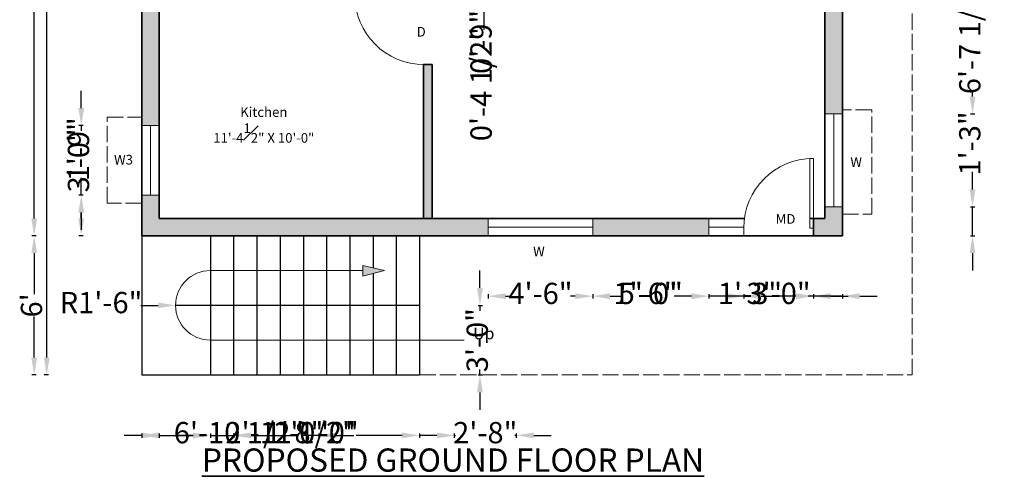
# Model space of a CAD drawing. Units: inches. Extents: x 2339 to 2848, y 489 to 1121.
# Tile 1 of 3: x 2339 to 2848, y 489 to 725. Entities that reach past the tile are written whole.
import ezdxf

# ---------------------------------------------------------------- set-up
doc = ezdxf.new("R2010")
doc.units = ezdxf.units.IN
doc.linetypes.add('ACAD_ISO02W100', pattern=[15, 12, -3])
for name, color, linetype, lineweight in [('A-ANNO-DIMS', 2, 'Continuous', 18), ('A-ANNO-SYMB', 7, 'Continuous', 18), ('A-ANNO-TEXT', 7, 'Continuous', 18), ('A-ANNO-TITL', 7, 'Continuous', 35), ('A-AREA-IDEN', 7, 'Continuous', 18), ('A-DOOR', 3, 'Continuous', 18), ('A-FLOR-STRS', 7, 'Continuous', 25), ('A-GLAZ', 4, 'Continuous', 18), ('A-ROOF-OVHD', 8, 'ACAD_ISO02W100', 13), ('A-WALL', 7, 'Continuous', 35), ('C-PROP', 8, 'ACAD_ISO02W100', 18)]:
    doc.layers.add(name, color=color, linetype=linetype, lineweight=lineweight)
doc.layers.add('A-WALL-PATT', color=18, linetype='Continuous', lineweight=13, true_color=0x000000)
doc.styles.get("Standard").update_dxf_attribs({"font": 'arial.ttf'})
doc.dimstyles.new('ISO-25', dxfattribs={"dimtxt": 11, "dimasz": 9, "dimexe": 1.25, "dimexo": 0.625, "dimtad": 0, "dimlunit": 4, "dimtxsty": 'Standard', "dimcen": 2.5, "dimadec": 0, "dimazin": 0, "dimtfac": 1, "dimtmove": 0, "dimatfit": 3, "dimfxl": 1, "dimfxlon": 1, "dimfrac": 1, "dimarcsym": 0})

# ---------------------------------------------------------------- blocks, each defined once
blk = doc.blocks.new('*U2')
for p, q in [((0, 0), (0, -4)), ((36, 0), (36, -4))]:
    blk.add_line(p, q)
blk.add_lwpolyline([(0, 0), (0, 36), (1.75, 36), (1.75, 0)], close=True)
blk.add_arc((0, 0), 36, 0, 90)
blk = doc.blocks.new('*D4')
at = {"layer": 'A-ANNO-DIMS', "color": 0, "lineweight": -2, "transparency": 16777216}
for p, q in [((2347.8, 1057.44), (2345.55, 1057.44)), ((2346.8, 1048.44), (2346.8, 845.39)), ((2346.8, 622.44), (2346.8, 825.48)), ((2347.8, 613.44), (2345.55, 613.44))]:
    blk.add_line(p, q, dxfattribs=at)
at = {"layer": 'A-ANNO-DIMS', "color": 0, "transparency": 16777216}
for points in [[(2345.3, 1048.44), (2348.3, 1048.44), (2346.8, 1057.44)], [(2345.3, 622.44), (2348.3, 622.44), (2346.8, 613.44)]]:
    blk.add_solid(points, dxfattribs=at)
at = {"layer": 'Defpoints', "color": 0, "transparency": 16777216}
for p in [(2402.35, 1057.44), (2346.8, 613.44), (2402.35, 613.44)]:
    blk.add_point(p, dxfattribs=at)
at = {"layer": 'A-ANNO-DIMS', "color": 0, "transparency": 16777216, "insert": (2346.8, 835.44), "char_height": 11, "attachment_point": 5, "rotation": 90}
blk.add_mtext("37'", dxfattribs=at)
blk = doc.blocks.new('*D5')
at = {"layer": 'A-ANNO-DIMS', "color": 0, "lineweight": -2, "transparency": 16777216}
for p, q in [((2347.8, 613.44), (2345.55, 613.44)), ((2346.8, 604.44), (2346.8, 583.15)), ((2346.8, 550.44), (2346.8, 571.72)), ((2347.8, 541.44), (2345.55, 541.44))]:
    blk.add_line(p, q, dxfattribs=at)
at = {"layer": 'A-ANNO-DIMS', "color": 0, "transparency": 16777216}
for points in [[(2345.3, 604.44), (2348.3, 604.44), (2346.8, 613.44)], [(2345.3, 550.44), (2348.3, 550.44), (2346.8, 541.44)]]:
    blk.add_solid(points, dxfattribs=at)
at = {"layer": 'Defpoints', "color": 0, "transparency": 16777216}
for p in [(2402.35, 613.44), (2346.8, 541.44), (2402.35, 541.44)]:
    blk.add_point(p, dxfattribs=at)
at = {"layer": 'A-ANNO-DIMS', "color": 0, "transparency": 16777216, "insert": (2346.8, 577.44), "char_height": 11, "attachment_point": 5, "rotation": 90}
blk.add_mtext("6'", dxfattribs=at)
blk = doc.blocks.new('WIN-48IN')
for p, q in [((0, 0), (0, 9)), ((48, 0), (48, 9)), ((0, 4.5), (48, 4.5))]:
    blk.add_line(p, q)
blk = doc.blocks.new('*D11')
at = {"layer": 'A-ANNO-DIMS', "color": 0, "lineweight": -2, "transparency": 16777216}
for p, q in [((2354.26, 1082.3), (2352.01, 1082.3)), ((2353.26, 1073.3), (2353.26, 831.61)), ((2353.26, 550.44), (2353.26, 792.13)), ((2354.26, 541.44), (2352.01, 541.44))]:
    blk.add_line(p, q, dxfattribs=at)
at = {"layer": 'A-ANNO-DIMS', "color": 0, "transparency": 16777216}
for points in [[(2351.76, 1073.3), (2354.76, 1073.3), (2353.26, 1082.3)], [(2351.76, 550.44), (2354.76, 550.44), (2353.26, 541.44)]]:
    blk.add_solid(points, dxfattribs=at)
at = {"layer": 'Defpoints', "color": 0, "transparency": 16777216}
for p in [(2353.26, 1082.3), (2493.85, 1082.3), (2402.35, 541.44)]:
    blk.add_point(p, dxfattribs=at)
at = {"layer": 'A-ANNO-DIMS', "color": 0, "transparency": 16777216, "insert": (2353.26, 811.87), "char_height": 11, "attachment_point": 5, "rotation": 90}
blk.add_mtext('45\'-1"', dxfattribs=at)
blk = doc.blocks.new('*D12')
at = {"layer": 'A-ANNO-DIMS', "color": 0, "lineweight": -2, "transparency": 16777216}
for p, q in [((2402.35, 511.19), (2402.35, 508.94)), ((2411.35, 510.19), (2428.85, 510.19)), ((2437.85, 511.19), (2437.85, 508.94)), ((2437.85, 510.19), (2446.85, 510.19))]:
    blk.add_line(p, q, dxfattribs=at)
at = {"layer": 'A-ANNO-DIMS', "color": 0, "transparency": 16777216}
for points in [[(2411.35, 511.69), (2411.35, 508.69), (2402.35, 510.19)], [(2428.85, 511.69), (2428.85, 508.69), (2437.85, 510.19)]]:
    blk.add_solid(points, dxfattribs=at)
at = {"layer": 'Defpoints', "color": 0, "transparency": 16777216}
for p in [(2402.35, 541.44), (2437.85, 541.44), (2437.85, 510.19)]:
    blk.add_point(p, dxfattribs=at)
at = {"layer": 'A-ANNO-DIMS', "color": 0, "transparency": 16777216, "insert": (2479.27, 510.19), "char_height": 11, "attachment_point": 5}
blk.add_mtext('2\'-11 1/2"', dxfattribs=at)
blk = doc.blocks.new('*D13')
at = {"layer": 'A-ANNO-DIMS', "color": 0, "lineweight": -2, "transparency": 16777216}
for p, q in [((2428.85, 510.19), (2419.85, 510.19)), ((2437.85, 511.19), (2437.85, 508.94)), ((2437.85, 510.19), (2449.85, 510.19)), ((2449.85, 511.19), (2449.85, 508.94)), ((2458.85, 510.19), (2467.85, 510.19))]:
    blk.add_line(p, q, dxfattribs=at)
at = {"layer": 'A-ANNO-DIMS', "color": 0, "transparency": 16777216}
for points in [[(2428.85, 511.69), (2428.85, 508.69), (2437.85, 510.19)], [(2458.85, 511.69), (2458.85, 508.69), (2449.85, 510.19)]]:
    blk.add_solid(points, dxfattribs=at)
at = {"layer": 'Defpoints', "color": 0, "transparency": 16777216}
for p in [(2437.85, 541.44), (2449.85, 541.44), (2449.85, 510.19)]:
    blk.add_point(p, dxfattribs=at)
at = {"layer": 'A-ANNO-DIMS', "color": 0, "transparency": 16777216, "insert": (2482.57, 510.19), "char_height": 11, "attachment_point": 5}
blk.add_mtext('1\'-0"', dxfattribs=at)
blk = doc.blocks.new('*D14')
at = {"layer": 'A-ANNO-DIMS', "color": 0, "lineweight": -2, "transparency": 16777216}
for p, q in [((2449.85, 511.19), (2449.85, 508.94)), ((2458.85, 510.19), (2482.59, 510.19)), ((2536.85, 510.19), (2513.1, 510.19)), ((2545.85, 511.19), (2545.85, 508.94))]:
    blk.add_line(p, q, dxfattribs=at)
at = {"layer": 'A-ANNO-DIMS', "color": 0, "transparency": 16777216}
for points in [[(2458.85, 511.69), (2458.85, 508.69), (2449.85, 510.19)], [(2536.85, 511.69), (2536.85, 508.69), (2545.85, 510.19)]]:
    blk.add_solid(points, dxfattribs=at)
at = {"layer": 'Defpoints', "color": 0, "transparency": 16777216}
for p in [(2449.85, 541.44), (2545.85, 541.44), (2545.85, 510.19)]:
    blk.add_point(p, dxfattribs=at)
at = {"layer": 'A-ANNO-DIMS', "color": 0, "transparency": 16777216, "insert": (2497.85, 510.19), "char_height": 11, "attachment_point": 5}
blk.add_mtext('8\'-0"', dxfattribs=at)
blk = doc.blocks.new('*D15')
at = {"layer": 'A-ANNO-DIMS', "color": 0, "lineweight": -2, "transparency": 16777216}
for p, q in [((2581.35, 583.19), (2581.35, 580.94)), ((2590.35, 582.19), (2592.88, 582.19)), ((2626.35, 582.19), (2623.81, 582.19)), ((2635.35, 583.19), (2635.35, 580.94))]:
    blk.add_line(p, q, dxfattribs=at)
at = {"layer": 'A-ANNO-DIMS', "color": 0, "transparency": 16777216}
for points in [[(2590.35, 583.69), (2590.35, 580.69), (2581.35, 582.19)], [(2626.35, 583.69), (2626.35, 580.69), (2635.35, 582.19)]]:
    blk.add_solid(points, dxfattribs=at)
at = {"layer": 'Defpoints', "color": 0, "transparency": 16777216}
for p in [(2581.35, 613.44), (2635.35, 613.44), (2581.35, 582.19)]:
    blk.add_point(p, dxfattribs=at)
at = {"layer": 'A-ANNO-DIMS', "color": 0, "transparency": 16777216, "insert": (2608.35, 582.19), "char_height": 11, "attachment_point": 5}
blk.add_mtext('4\'-6"', dxfattribs=at)
blk = doc.blocks.new('*D16')
at = {"layer": 'A-ANNO-DIMS', "color": 0, "lineweight": -2, "transparency": 16777216}
for p, q in [((2635.35, 583.19), (2635.35, 580.94)), ((2644.35, 582.19), (2650.1, 582.19)), ((2686.35, 582.19), (2680.59, 582.19)), ((2695.35, 583.19), (2695.35, 580.94))]:
    blk.add_line(p, q, dxfattribs=at)
at = {"layer": 'A-ANNO-DIMS', "color": 0, "transparency": 16777216}
for points in [[(2644.35, 583.69), (2644.35, 580.69), (2635.35, 582.19)], [(2686.35, 583.69), (2686.35, 580.69), (2695.35, 582.19)]]:
    blk.add_solid(points, dxfattribs=at)
at = {"layer": 'Defpoints', "color": 0, "transparency": 16777216}
for p in [(2635.35, 613.44), (2695.35, 613.44), (2635.35, 582.19)]:
    blk.add_point(p, dxfattribs=at)
at = {"layer": 'A-ANNO-DIMS', "color": 0, "transparency": 16777216, "insert": (2665.35, 582.19), "char_height": 11, "attachment_point": 5}
blk.add_mtext('5\'-0"', dxfattribs=at)
blk = doc.blocks.new('*D17')
at = {"layer": 'A-ANNO-DIMS', "color": 0, "lineweight": -2, "transparency": 16777216}
for p, q in [((2686.35, 582.19), (2677.35, 582.19)), ((2695.35, 583.19), (2695.35, 580.94)), ((2713.35, 582.19), (2695.35, 582.19)), ((2713.35, 583.19), (2713.35, 580.94)), ((2722.35, 582.19), (2731.35, 582.19))]:
    blk.add_line(p, q, dxfattribs=at)
at = {"layer": 'A-ANNO-DIMS', "color": 0, "transparency": 16777216}
for points in [[(2686.35, 583.69), (2686.35, 580.69), (2695.35, 582.19)], [(2722.35, 583.69), (2722.35, 580.69), (2713.35, 582.19)]]:
    blk.add_solid(points, dxfattribs=at)
at = {"layer": 'Defpoints', "color": 0, "transparency": 16777216}
for p in [(2695.35, 613.44), (2713.35, 613.44), (2695.35, 582.19)]:
    blk.add_point(p, dxfattribs=at)
at = {"layer": 'A-ANNO-DIMS', "color": 0, "transparency": 16777216, "insert": (2662.62, 582.19), "char_height": 11, "attachment_point": 5}
blk.add_mtext('1\'-6"', dxfattribs=at)
blk = doc.blocks.new('*D18')
at = {"layer": 'A-ANNO-DIMS', "color": 0, "lineweight": -2, "transparency": 16777216}
for p, q in [((2704.35, 582.19), (2695.35, 582.19)), ((2713.35, 583.19), (2713.35, 580.94)), ((2713.35, 582.19), (2716.11, 582.19)), ((2749.35, 582.19), (2746.59, 582.19)), ((2749.35, 583.19), (2749.35, 580.94)), ((2758.35, 582.19), (2767.35, 582.19))]:
    blk.add_line(p, q, dxfattribs=at)
at = {"layer": 'A-ANNO-DIMS', "color": 0, "transparency": 16777216}
for points in [[(2704.35, 583.69), (2704.35, 580.69), (2713.35, 582.19)], [(2758.35, 583.69), (2758.35, 580.69), (2749.35, 582.19)]]:
    blk.add_solid(points, dxfattribs=at)
at = {"layer": 'Defpoints', "color": 0, "transparency": 16777216}
for p in [(2713.35, 613.44), (2749.35, 613.44), (2713.35, 582.19)]:
    blk.add_point(p, dxfattribs=at)
at = {"layer": 'A-ANNO-DIMS', "color": 0, "transparency": 16777216, "insert": (2731.35, 582.19), "char_height": 11, "attachment_point": 5}
blk.add_mtext('3\'-0"', dxfattribs=at)
blk = doc.blocks.new('*D19')
at = {"layer": 'A-ANNO-DIMS', "color": 0, "lineweight": -2, "transparency": 16777216}
for p, q in [((2740.35, 582.19), (2731.35, 582.19)), ((2749.35, 583.19), (2749.35, 580.94)), ((2764.35, 582.19), (2749.35, 582.19)), ((2764.35, 583.19), (2764.35, 580.94)), ((2773.35, 582.19), (2782.35, 582.19))]:
    blk.add_line(p, q, dxfattribs=at)
at = {"layer": 'A-ANNO-DIMS', "color": 0, "transparency": 16777216}
for points in [[(2740.35, 583.69), (2740.35, 580.69), (2749.35, 582.19)], [(2773.35, 583.69), (2773.35, 580.69), (2764.35, 582.19)]]:
    blk.add_solid(points, dxfattribs=at)
at = {"layer": 'Defpoints', "color": 0, "transparency": 16777216}
for p in [(2749.35, 613.44), (2764.35, 613.44), (2749.35, 582.19)]:
    blk.add_point(p, dxfattribs=at)
at = {"layer": 'A-ANNO-DIMS', "color": 0, "transparency": 16777216, "insert": (2716.62, 582.19), "char_height": 11, "attachment_point": 5}
blk.add_mtext('1\'-3"', dxfattribs=at)
blk = doc.blocks.new('*D20')
at = {"layer": 'A-ANNO-DIMS', "color": 0, "lineweight": -2, "transparency": 16777216}
for p, q in [((2371.1, 634.44), (2371.1, 643.44)), ((2372.1, 634.44), (2369.85, 634.44)), ((2371.1, 622.44), (2371.1, 625.44)), ((2372.1, 613.44), (2369.85, 613.44))]:
    blk.add_line(p, q, dxfattribs=at)
at = {"layer": 'A-ANNO-DIMS', "color": 0, "transparency": 16777216}
for points in [[(2369.6, 625.44), (2372.6, 625.44), (2371.1, 634.44)], [(2369.6, 622.44), (2372.6, 622.44), (2371.1, 613.44)]]:
    blk.add_solid(points, dxfattribs=at)
at = {"layer": 'Defpoints', "color": 0, "transparency": 16777216}
for p in [(2371.1, 634.44), (2402.35, 634.44), (2402.35, 613.44)]:
    blk.add_point(p, dxfattribs=at)
at = {"layer": 'A-ANNO-DIMS', "color": 0, "transparency": 16777216, "insert": (2371.1, 658.17), "char_height": 11, "attachment_point": 5, "rotation": 90}
blk.add_mtext('1\'-9"', dxfattribs=at)
blk = doc.blocks.new('*D21')
at = {"layer": 'A-ANNO-DIMS', "color": 0, "lineweight": -2, "transparency": 16777216}
for p, q in [((2371.1, 679.44), (2371.1, 688.44)), ((2372.1, 670.44), (2369.85, 670.44)), ((2371.1, 670.44), (2371.1, 667.68)), ((2371.1, 634.44), (2371.1, 637.2)), ((2372.1, 634.44), (2369.85, 634.44)), ((2371.1, 625.44), (2371.1, 616.44))]:
    blk.add_line(p, q, dxfattribs=at)
at = {"layer": 'A-ANNO-DIMS', "color": 0, "transparency": 16777216}
for points in [[(2369.6, 679.44), (2372.6, 679.44), (2371.1, 670.44)], [(2369.6, 625.44), (2372.6, 625.44), (2371.1, 634.44)]]:
    blk.add_solid(points, dxfattribs=at)
at = {"layer": 'Defpoints', "color": 0, "transparency": 16777216}
for p in [(2371.1, 670.44), (2402.35, 670.44), (2402.35, 634.44)]:
    blk.add_point(p, dxfattribs=at)
at = {"layer": 'A-ANNO-DIMS', "color": 0, "transparency": 16777216, "insert": (2371.1, 652.44), "char_height": 11, "attachment_point": 5, "rotation": 90}
blk.add_mtext('3\'-0"', dxfattribs=at)
blk = doc.blocks.new('*D27')
at = {"layer": 'A-ANNO-DIMS', "color": 0, "lineweight": -2, "transparency": 16777216}
for p, q in [((2402.35, 510.19), (2393.35, 510.19)), ((2411.35, 511.19), (2411.35, 508.94)), ((2411.35, 510.19), (2420.23, 510.19)), ((2493.85, 510.19), (2484.96, 510.19)), ((2493.85, 511.19), (2493.85, 508.94)), ((2502.85, 510.19), (2511.85, 510.19))]:
    blk.add_line(p, q, dxfattribs=at)
at = {"layer": 'A-ANNO-DIMS', "color": 0, "transparency": 16777216}
for points in [[(2402.35, 511.69), (2402.35, 508.69), (2411.35, 510.19)], [(2502.85, 511.69), (2502.85, 508.69), (2493.85, 510.19)]]:
    blk.add_solid(points, dxfattribs=at)
at = {"layer": 'Defpoints', "color": 0, "transparency": 16777216}
for p in [(2411.35, 1048.44), (2493.85, 1048.44), (2493.85, 510.19)]:
    blk.add_point(p, dxfattribs=at)
at = {"layer": 'A-ANNO-DIMS', "color": 0, "transparency": 16777216, "insert": (2452.6, 510.19), "char_height": 11, "attachment_point": 5}
blk.add_mtext('6\'-10 1/2"', dxfattribs=at)
blk = doc.blocks.new('*D31')
at = {"layer": 'A-ANNO-DIMS', "color": 0, "lineweight": -2, "transparency": 16777216}
for p, q in [((2831.6, 637.44), (2831.6, 646.44)), ((2830.6, 628.44), (2832.85, 628.44)), ((2831.6, 613.44), (2831.6, 628.44)), ((2830.6, 613.44), (2832.85, 613.44)), ((2831.6, 604.44), (2831.6, 595.44))]:
    blk.add_line(p, q, dxfattribs=at)
at = {"layer": 'A-ANNO-DIMS', "color": 0, "transparency": 16777216}
for points in [[(2830.1, 637.44), (2833.1, 637.44), (2831.6, 628.44)], [(2830.1, 604.44), (2833.1, 604.44), (2831.6, 613.44)]]:
    blk.add_solid(points, dxfattribs=at)
at = {"layer": 'Defpoints', "color": 0, "transparency": 16777216}
for p in [(2764.35, 628.44), (2831.6, 628.44), (2764.35, 613.44)]:
    blk.add_point(p, dxfattribs=at)
at = {"layer": 'A-ANNO-DIMS', "color": 0, "transparency": 16777216, "insert": (2831.6, 661.17), "char_height": 11, "attachment_point": 5, "rotation": 90}
blk.add_mtext('1\'-3"', dxfattribs=at)
blk = doc.blocks.new('*D32')
at = {"layer": 'A-ANNO-DIMS', "color": 0, "lineweight": -2, "transparency": 16777216}
for p, q in [((2830.6, 755.94), (2832.85, 755.94)), ((2831.6, 746.94), (2831.6, 744.28)), ((2831.6, 685.44), (2831.6, 688.1)), ((2830.6, 676.44), (2832.85, 676.44))]:
    blk.add_line(p, q, dxfattribs=at)
at = {"layer": 'A-ANNO-DIMS', "color": 0, "transparency": 16777216}
for points in [[(2830.1, 746.94), (2833.1, 746.94), (2831.6, 755.94)], [(2830.1, 685.44), (2833.1, 685.44), (2831.6, 676.44)]]:
    blk.add_solid(points, dxfattribs=at)
at = {"layer": 'Defpoints', "color": 0, "transparency": 16777216}
for p in [(2764.35, 755.94), (2831.6, 755.94), (2764.35, 676.44)]:
    blk.add_point(p, dxfattribs=at)
at = {"layer": 'A-ANNO-DIMS', "color": 0, "transparency": 16777216, "insert": (2831.6, 716.19), "char_height": 11, "attachment_point": 5, "rotation": 90}
blk.add_mtext('6\'-7 1/2"', dxfattribs=at)
blk = doc.blocks.new('*D36')
at = {"layer": 'A-ANNO-DIMS', "color": 0, "lineweight": -2, "transparency": 16777216}
for p, q in [((2554.85, 510.19), (2545.85, 510.19)), ((2563.85, 511.19), (2563.85, 508.94)), ((2563.85, 510.19), (2564.51, 510.19)), ((2595.85, 510.19), (2595.19, 510.19)), ((2595.85, 511.19), (2595.85, 508.94)), ((2604.85, 510.19), (2613.85, 510.19))]:
    blk.add_line(p, q, dxfattribs=at)
at = {"layer": 'A-ANNO-DIMS', "color": 0, "transparency": 16777216}
for points in [[(2554.85, 511.69), (2554.85, 508.69), (2563.85, 510.19)], [(2604.85, 511.69), (2604.85, 508.69), (2595.85, 510.19)]]:
    blk.add_solid(points, dxfattribs=at)
at = {"layer": 'Defpoints', "color": 0, "transparency": 16777216}
for p in [(2563.85, 971.94), (2595.85, 971.94), (2595.85, 510.19)]:
    blk.add_point(p, dxfattribs=at)
at = {"layer": 'A-ANNO-DIMS', "color": 0, "transparency": 16777216, "insert": (2579.85, 510.19), "char_height": 11, "attachment_point": 5}
blk.add_mtext('2\'-8"', dxfattribs=at)
blk = doc.blocks.new('*D41')
at = {"layer": 'A-ANNO-DIMS', "color": 0, "lineweight": -2, "transparency": 16777216}
for p, q in [((2577.1, 586.44), (2577.1, 595.44)), ((2576.1, 577.44), (2578.35, 577.44)), ((2577.1, 577.44), (2577.1, 574.68)), ((2576.1, 541.44), (2578.35, 541.44)), ((2577.1, 541.44), (2577.1, 544.2)), ((2577.1, 532.44), (2577.1, 523.44))]:
    blk.add_line(p, q, dxfattribs=at)
at = {"layer": 'A-ANNO-DIMS', "color": 0, "transparency": 16777216}
for points in [[(2575.6, 586.44), (2578.6, 586.44), (2577.1, 577.44)], [(2575.6, 532.44), (2578.6, 532.44), (2577.1, 541.44)]]:
    blk.add_solid(points, dxfattribs=at)
at = {"layer": 'Defpoints', "color": 0, "transparency": 16777216}
for p in [(2545.85, 577.44), (2545.85, 541.44), (2577.1, 541.44)]:
    blk.add_point(p, dxfattribs=at)
at = {"layer": 'A-ANNO-DIMS', "color": 0, "transparency": 16777216, "insert": (2577.1, 559.44), "char_height": 11, "attachment_point": 5, "rotation": 90}
blk.add_mtext('3\'-0"', dxfattribs=at)
blk = doc.blocks.new('*D45')
at = {"layer": 'A-ANNO-DIMS', "color": 0, "lineweight": -2, "transparency": 16777216}
for p, q in [((2579.1, 764.94), (2579.1, 773.94)), ((2578.1, 755.94), (2580.35, 755.94)), ((2579.1, 755.94), (2579.1, 746.94)), ((2578.1, 746.94), (2580.35, 746.94)), ((2579.1, 737.94), (2579.1, 728.94))]:
    blk.add_line(p, q, dxfattribs=at)
at = {"layer": 'A-ANNO-DIMS', "color": 0, "transparency": 16777216}
for points in [[(2577.6, 764.94), (2580.6, 764.94), (2579.1, 755.94)], [(2577.6, 737.94), (2580.6, 737.94), (2579.1, 746.94)]]:
    blk.add_solid(points, dxfattribs=at)
at = {"layer": 'Defpoints', "color": 0, "transparency": 16777216}
for p in [(2547.85, 755.94), (2547.85, 746.94), (2579.1, 746.94)]:
    blk.add_point(p, dxfattribs=at)
at = {"layer": 'A-ANNO-DIMS', "color": 0, "transparency": 16777216, "insert": (2579.1, 713.69), "char_height": 11, "attachment_point": 5, "rotation": 90}
blk.add_mtext('0\'-9"', dxfattribs=at)
blk = doc.blocks.new('*D46')
at = {"layer": 'A-ANNO-DIMS', "color": 0, "lineweight": -2, "transparency": 16777216}
for p, q in [((2579.1, 751.44), (2579.1, 760.44)), ((2578.1, 742.44), (2580.35, 742.44)), ((2578.1, 737.94), (2580.35, 737.94)), ((2579.1, 742.44), (2579.1, 737.94)), ((2579.1, 728.94), (2579.1, 719.94))]:
    blk.add_line(p, q, dxfattribs=at)
at = {"layer": 'A-ANNO-DIMS', "color": 0, "transparency": 16777216}
for points in [[(2577.6, 751.44), (2580.6, 751.44), (2579.1, 742.44)], [(2577.6, 728.94), (2580.6, 728.94), (2579.1, 737.94)]]:
    blk.add_solid(points, dxfattribs=at)
at = {"layer": 'Defpoints', "color": 0, "transparency": 16777216}
for p in [(2547.85, 742.44), (2547.85, 737.94), (2579.1, 737.94)]:
    blk.add_point(p, dxfattribs=at)
at = {"layer": 'A-ANNO-DIMS', "color": 0, "transparency": 16777216, "insert": (2579.1, 691.88), "char_height": 11, "attachment_point": 5, "rotation": 90}
blk.add_mtext('0\'-4 1/2"', dxfattribs=at)
blk = doc.blocks.new('*D48')
at = {"layer": 'A-ANNO-DIMS', "color": 0, "lineweight": -2, "transparency": 16777216}
for p, q in [((2401.85, 577.44), (2410.85, 577.44)), ((2437.85, 577.44), (2419.85, 577.44))]:
    blk.add_line(p, q, dxfattribs=at)
at = {"layer": 'A-ANNO-DIMS', "color": 0, "transparency": 16777216}
blk.add_solid([(2410.85, 578.94), (2410.85, 575.94), (2419.85, 577.44)], dxfattribs=at)
at = {"layer": 'Defpoints', "color": 0, "transparency": 16777216}
for p in [(2419.85, 577.44), (2437.85, 577.44)]:
    blk.add_point(p, dxfattribs=at)
at = {"layer": 'A-ANNO-DIMS', "color": 0, "transparency": 16777216, "insert": (2381.34, 577.44), "char_height": 11, "attachment_point": 5, "rotation": 359.9991}
blk.add_mtext('R1\'-6"', dxfattribs=at)

msp = doc.modelspace()

# ---------------------------------------------------------------- hatches: boundary and pattern name
at = {"layer": 'A-ANNO-SYMB'}
h = msp.add_hatch(color=256, dxfattribs=at)
h.dxf.hatch_style = 1
h.paths.add_polyline_path([(2516.636, 597.983), (2516.636, 592.471), (2527.847, 595.438)])
at = {"layer": 'A-WALL-PATT'}
h = msp.add_hatch(color=256, dxfattribs=at)
h.dxf.hatch_style = 1
h.paths.add_polyline_path([(2493.847, 1057.438), (2402.347, 1057.438), (2402.347, 991.938), (2411.347, 991.938), (2411.347, 1048.438), (2493.847, 1048.438)])
h.paths.add_polyline_path([(2411.347, 931.938), (2402.347, 931.938), (2402.347, 912.438), (2411.347, 912.438), (2411.347, 918.438)])
h.paths.add_polyline_path([(2411.347, 871.438), (2411.347, 877.438), (2402.347, 877.438), (2402.347, 803.938), (2411.347, 803.938)])
h.paths.add_polyline_path([(2547.847, 871.438), (2411.347, 871.438), (2411.347, 866.938), (2547.847, 866.938)])
h.paths.add_polyline_path([(2447.347, 922.938), (2411.347, 922.938), (2411.347, 918.438), (2447.347, 918.438)])
h.paths.add_polyline_path([(2552.347, 866.938), (2547.847, 866.938), (2547.847, 791.938), (2552.347, 791.938)])
h.paths.add_polyline_path([(2411.347, 755.938), (2402.347, 755.938), (2402.347, 670.438), (2411.347, 670.438)])
h.paths.add_polyline_path([(2552.347, 755.938), (2547.847, 755.938), (2547.847, 746.938), (2411.347, 746.938), (2411.347, 742.438), (2547.847, 742.438), (2547.847, 737.938), (2552.347, 737.938)])
h.paths.add_polyline_path([(2552.347, 701.938), (2547.847, 701.938), (2547.847, 622.438), (2552.347, 622.438)])
h.paths.add_polyline_path([(2581.347, 622.438), (2411.347, 622.438), (2411.347, 634.438), (2402.347, 634.438), (2402.347, 613.438), (2581.347, 613.438)])
h.paths.add_polyline_path([(2695.347, 622.438), (2635.347, 622.438), (2635.347, 613.438), (2695.347, 613.438)])
h.paths.add_polyline_path([(2764.347, 628.438), (2755.347, 628.438), (2755.347, 622.438), (2749.347, 622.438), (2749.347, 613.438), (2764.347, 613.438)])
h.paths.add_polyline_path([(2764.347, 755.938), (2760.347, 755.938), (2755.347, 755.938), (2755.347, 676.438), (2764.347, 676.438)])
h.paths.add_polyline_path([(2764.347, 931.938), (2755.347, 931.938), (2755.347, 851.938), (2764.347, 851.938)])
h.paths.add_polyline_path([(2764.347, 1057.438), (2749.347, 1057.438), (2749.347, 1048.438), (2755.347, 1048.438), (2755.347, 979.938), (2764.347, 979.938)])
h.paths.add_polyline_path([(2701.347, 1057.438), (2594.347, 1057.438), (2594.347, 1048.438), (2604.847, 1048.438), (2701.347, 1048.438)])
h.paths.add_polyline_path([(2558.347, 1057.438), (2541.847, 1057.438), (2541.847, 1048.438), (2552.347, 1048.438), (2558.347, 1048.438)])

# ---------------------------------------------------------------- linework, layer by layer
at = {"layer": 'A-ANNO-SYMB'}
for p, q in [((2516.636, 595.438), (2437.847, 595.438)), ((2516.636, 597.983), (2516.636, 592.471)), ((2527.847, 595.438), (2516.636, 597.983)), ((2516.636, 592.471), (2527.847, 595.438)), ((2437.847, 559.438), (2568.925, 559.438))]:
    msp.add_line(p, q, dxfattribs=at)
msp.add_arc((2437.847, 577.438), 18, 90, 270, dxfattribs=at)
at = {"layer": 'A-FLOR-STRS'}
for p, q in [((2402.347, 613.438), (2402.347, 541.438)), ((2437.847, 613.438), (2437.847, 541.438)), ((2449.847, 613.438), (2449.847, 541.438)), ((2461.847, 613.438), (2461.847, 541.438)), ((2473.847, 613.438), (2473.847, 541.438)), ((2485.847, 613.438), (2485.847, 541.438)), ((2497.847, 613.438), (2497.847, 541.438)), ((2509.847, 613.438), (2509.847, 541.438)), ((2521.847, 613.438), (2521.847, 596.8)), ((2533.847, 613.438), (2533.847, 541.438)), ((2545.847, 613.438), (2545.847, 541.438)), ((2521.847, 593.85), (2521.847, 541.438)), ((2545.847, 577.438), (2437.847, 577.438)), ((2402.347, 541.438), (2545.847, 541.438))]:
    msp.add_line(p, q, dxfattribs=at)
at = {"layer": 'A-GLAZ'}
for p, q in [((2402.347, 670.438), (2411.347, 670.438)), ((2406.847, 634.438), (2406.847, 670.438)), ((2402.347, 634.438), (2411.347, 634.438)), ((2581.347, 613.438), (2581.347, 622.438)), ((2635.347, 613.438), (2635.347, 622.438)), ((2695.347, 613.438), (2695.347, 622.438)), ((2581.347, 617.938), (2635.347, 617.938)), ((2695.347, 617.938), (2713.347, 617.938))]:
    msp.add_line(p, q, dxfattribs=at)
at = {"layer": 'A-ROOF-OVHD', "ltscale": 0.7}
for p, q in [((2779.567, 678.532), (2764.347, 678.532)), ((2779.567, 624.672), (2779.567, 678.532)), ((2384.51, 630.362), (2384.51, 674.815)), ((2384.51, 674.815), (2402.347, 674.815)), ((2402.347, 630.362), (2384.51, 630.362)), ((2764.347, 624.672), (2779.567, 624.672))]:
    msp.add_line(p, q, dxfattribs=at)
at = {"layer": 'A-WALL'}
for p, q in [((2402.347, 1057.438), (2402.347, 613.438)), ((2411.347, 871.438), (2411.347, 622.438)), ((2764.347, 613.438), (2764.347, 791.938)), ((2755.347, 622.438), (2755.347, 757.688)), ((2547.847, 701.938), (2552.347, 701.938)), ((2547.847, 701.938), (2547.847, 622.438)), ((2552.347, 701.938), (2552.347, 622.438)), ((2411.347, 622.438), (2713.696, 622.438)), ((2747.597, 622.438), (2755.347, 622.438)), ((2749.347, 622.438), (2749.347, 613.438)), ((2402.347, 613.438), (2749.347, 613.438)), ((2749.347, 613.438), (2764.347, 613.438))]:
    msp.add_line(p, q, dxfattribs=at)
at = {"layer": 'C-PROP', "ltscale": 0.7}
for p, q in [((2800.347, 541.438), (2800.347, 1057.438)), ((2545.847, 541.438), (2800.347, 541.438))]:
    msp.add_line(p, q, dxfattribs=at)

# ---------------------------------------------------------------- block references
at = {"layer": 'A-DOOR', "xscale": -1, "rotation": 90}
msp.add_blockref('*U2', (2548.347, 737.938), dxfattribs=at)
at = {"layer": 'A-DOOR', "xscale": -1}
msp.add_blockref('*U2', (2749.347, 617.438), dxfattribs=at)
at = {"layer": 'A-GLAZ', "rotation": 270.0000000000016}
msp.add_blockref('WIN-48IN', (2755.347, 676.438), dxfattribs=at)

# ---------------------------------------------------------------- texts
at = {"layer": 'A-ANNO-TEXT', "attachment_point": 1}
for s, width, insert, char_height in [('\\pxqc;D', 14.23587, (2539.621, 721.429), 5), ('\\pxqc;MD', 14.23587, (2727.84, 624.624), 5), ('\\pxqc;W', 14.23587, (2600.439, 607.803), 5), ('Up', 35.25998, (2573.593, 565.882), 6)]:
    msp.add_mtext_dynamic_manual_height_columns(s, width=width, gutter_width=12.5, heights=[0], dxfattribs=dict(at, insert=insert, char_height=char_height))
at = {"layer": 'A-ANNO-TEXT', "ltscale": 0.7, "char_height": 5, "attachment_point": 1}
for s, insert in [('\\pxqc;W3', (2385.825, 655.265)), ('\\pxqc;W', (2764.347, 654.037))]:
    msp.add_mtext_dynamic_manual_height_columns(s, width=14.23587, gutter_width=12.5, heights=[0], dxfattribs=dict(at, insert=insert))
at = {"layer": 'A-ANNO-TITL', "insert": (2433.407, 503.425), "char_height": 12, "attachment_point": 1}
msp.add_mtext_dynamic_manual_height_columns('{\\fArial|b1|i0|c0|p34;\\LPROPOSED GROUND FLOOR PLAN}', width=344.34832, gutter_width=12.5, heights=[0], dxfattribs=at)
at = {"layer": 'A-AREA-IDEN', "insert": (2416.805, 679.905), "char_height": 5, "attachment_point": 1}
msp.add_mtext_dynamic_manual_height_columns('\\pxqc;Kitchen\\P11\'-4\\S1#2;" X 10\'-0"', width=97.24493, gutter_width=12.5, heights=[0], dxfattribs=at)

# ---------------------------------------------------------------- dimensions: what is measured, and where the dimension line sits
at = {"layer": 'A-ANNO-DIMS'}
for base, p1, p2, angle, override, picture, middle in [((2353.26, 1082.304), (2402.347, 541.438), (2493.847, 1082.304), 90, {"dimdec": 1, "dimlfac": 1, "dimrnd": 0, "dimzin": 1, "dimdsep": 46, "dimlunit": 4, "dimfrac": 2}, '*D11', (2353.26, 811.871)), ((2346.8, 613.438), (2402.347, 1057.438), (2402.347, 613.438), 90, {"dimclrd": 0, "dimclre": 0, "dimclrt": 0}, '*D4', (2346.8, 835.438)), ((2579.097, 746.938), (2547.847, 755.938), (2547.847, 746.938), 270, {"dimdec": 1, "dimlfac": 1, "dimrnd": 0, "dimzin": 1, "dimdsep": 46, "dimlunit": 4, "dimfrac": 2}, '*D45', (2579.097, 713.692)), ((2579.097, 737.938), (2547.847, 742.438), (2547.847, 737.938), 270, {"dimdec": 1, "dimlfac": 1, "dimrnd": 0, "dimzin": 1, "dimdsep": 46, "dimlunit": 4, "dimfrac": 2}, '*D46', (2579.097, 691.876)), ((2831.597, 755.938), (2764.347, 676.438), (2764.347, 755.938), 90, {"dimdec": 1, "dimlfac": 1, "dimrnd": 0, "dimzin": 1, "dimdsep": 46, "dimlunit": 4, "dimfrac": 2}, '*D32', (2831.597, 716.188)), ((2371.097, 670.438), (2402.347, 634.438), (2402.347, 670.438), 90, {"dimdec": 1, "dimlfac": 1, "dimrnd": 0, "dimzin": 1, "dimdsep": 46, "dimlunit": 4, "dimfrac": 2}, '*D21', (2371.097, 652.438)), ((2831.597, 628.438), (2764.347, 613.438), (2764.347, 628.438), 90, {"dimdec": 1, "dimlfac": 1, "dimrnd": 0, "dimzin": 1, "dimdsep": 46, "dimlunit": 4, "dimfrac": 2}, '*D31', (2831.597, 661.165)), ((2371.097, 634.438), (2402.347, 613.438), (2402.347, 634.438), 90, {"dimdec": 1, "dimlfac": 1, "dimrnd": 0, "dimzin": 1, "dimdsep": 46, "dimlunit": 4, "dimfrac": 2}, '*D20', (2371.097, 658.165)), ((2346.8, 541.438), (2402.347, 613.438), (2402.347, 541.438), 90, {"dimclrd": 0, "dimclre": 0, "dimclrt": 0, "dimtmove": 1}, '*D5', (2346.8, 577.438)), ((2581.347, 582.188), (2635.347, 613.438), (2581.347, 613.438), 180, {"dimdec": 1, "dimlfac": 1, "dimrnd": 0, "dimzin": 1, "dimdsep": 46, "dimlunit": 4, "dimfrac": 2}, '*D15', (2608.347, 582.188)), ((2635.347, 582.188), (2695.347, 613.438), (2635.347, 613.438), 180, {"dimdec": 1, "dimlfac": 1, "dimrnd": 0, "dimzin": 1, "dimdsep": 46, "dimlunit": 4, "dimfrac": 2}, '*D16', (2665.347, 582.188)), ((2695.347, 582.188), (2713.347, 613.438), (2695.347, 613.438), 180, {"dimdec": 1, "dimlfac": 1, "dimrnd": 0, "dimzin": 1, "dimdsep": 46, "dimlunit": 4, "dimfrac": 2}, '*D17', (2662.619, 582.188)), ((2713.347, 582.188), (2749.347, 613.438), (2713.347, 613.438), 180, {"dimdec": 1, "dimlfac": 1, "dimrnd": 0, "dimzin": 1, "dimdsep": 46, "dimlunit": 4, "dimfrac": 2}, '*D18', (2731.347, 582.188)), ((2749.347, 582.188), (2764.347, 613.438), (2749.347, 613.438), 180, {"dimdec": 1, "dimlfac": 1, "dimrnd": 0, "dimzin": 1, "dimdsep": 46, "dimlunit": 4, "dimfrac": 2}, '*D19', (2716.619, 582.188)), ((2577.097, 541.438), (2545.847, 577.438), (2545.847, 541.438), 270, {"dimdec": 1, "dimlfac": 1, "dimrnd": 0, "dimzin": 1, "dimdsep": 46, "dimlunit": 4, "dimfrac": 2}, '*D41', (2577.097, 559.438))]:
    dim = msp.add_linear_dim(base=base, p1=p1, p2=p2, angle=angle, dimstyle='ISO-25', override=override, dxfattribs=at)
    dim.commit()
    dim.dimension.update_dxf_attribs({"geometry": picture, "text_midpoint": middle})
for base, p1, p2, picture, middle in [((2493.847, 510.188), (2411.347, 1048.438), (2493.847, 1048.438), '*D27', (2452.597, 510.188)), ((2595.847, 510.188), (2563.847, 971.938), (2595.847, 971.938), '*D36', (2579.847, 510.188)), ((2437.847, 510.188), (2402.347, 541.438), (2437.847, 541.438), '*D12', (2479.275, 510.188)), ((2449.847, 510.188), (2437.847, 541.438), (2449.847, 541.438), '*D13', (2482.574, 510.188)), ((2545.847, 510.188), (2449.847, 541.438), (2545.847, 541.438), '*D14', (2497.847, 510.188))]:
    dim = msp.add_linear_dim(base=base, p1=p1, p2=p2, dimstyle='ISO-25', override={"dimdec": 1, "dimlfac": 1, "dimrnd": 0, "dimzin": 1, "dimdsep": 46, "dimlunit": 4, "dimfrac": 2}, dxfattribs=at)
    dim.commit()
    dim.dimension.update_dxf_attribs({"geometry": picture, "text_midpoint": middle})
dim = msp.add_radius_dim(center=(2437.847, 577.438), mpoint=(2419.847, 577.438), dimstyle='ISO-25', override={"dimdec": 1, "dimlfac": 1, "dimrnd": 0, "dimzin": 1, "dimdsep": 46, "dimlunit": 4, "dimfrac": 2}, dxfattribs=at)
dim.commit()
dim.dimension.update_dxf_attribs({"geometry": '*D48', "text_midpoint": (2381.338, 577.439)})

doc.saveas('drawing.dxf')
